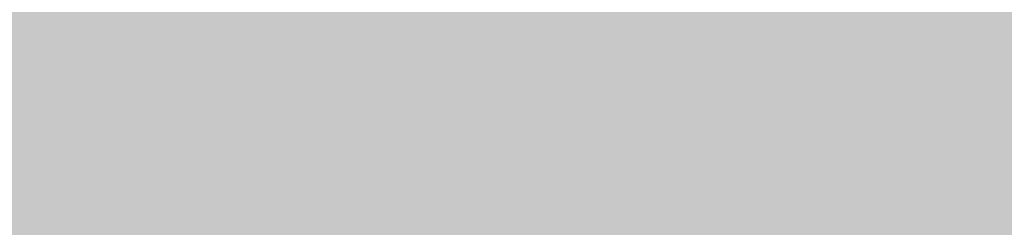
# Model space of a CAD drawing. Units: feet. Extents: x 3168 to 4724, y 827 to 1477.
# Tile 51 of 256: x 3273.0722 to 3273.13944, y 1099.00068 to 1099.01485. Entities that reach past the tile are written whole.
import ezdxf

# ---------------------------------------------------------------- set-up
doc = ezdxf.new("R2010")
doc.units = ezdxf.units.FT
doc.layers.add('A-ELEV', color=7, linetype='Continuous', lineweight=35)
doc.layers.add('A-ELEV-PATT', color=8, linetype='Continuous', lineweight=13)

msp = doc.modelspace()

# ---------------------------------------------------------------- hatches: boundary and pattern name
at = {"layer": 'A-ELEV-PATT'}
h = msp.add_hatch(color=256, dxfattribs=at)
h.dxf.hatch_style = 1
edge = h.paths.add_edge_path()
edge.add_ellipse((3552.905762, 979.220141), major_axis=(36.744924, 0), ratio=0.484848485, start_angle=0, end_angle=360)
edge = h.paths.add_edge_path()
edge.add_ellipse((3559.891637, 929.252282), major_axis=(36.744924, 0), ratio=0.484848485, start_angle=0, end_angle=360)
edge = h.paths.add_edge_path()
edge.add_line((3299.31681, 1198.606081), (3479.916714, 1198.606081))
edge.add_line((3479.916714, 1198.606081), (3479.916714, 1209.86857))
edge.add_spline(control_points=[(3479.916714, 1209.86857), (3464.301157, 1209.86857), (3448.685601, 1209.86857), (3410.949139, 1209.86857), (3388.828234, 1209.86857), (3355.646876, 1209.86857), (3344.586423, 1209.86857), (3327.995745, 1209.86857), (3322.465518, 1209.86857), (3314.170179, 1209.86857), (3311.405066, 1209.86857), (3307.257396, 1209.86857), (3305.874839, 1209.86857), (3303.801005, 1209.86857), (3303.109726, 1209.86857), (3302.072809, 1209.86857), (3301.72717, 1209.86857), (3301.208711, 1209.86857), (3301.035891, 1209.86857), (3300.776662, 1209.86857), (3300.690252, 1209.86857), (3300.560638, 1209.86857), (3300.517433, 1209.86857), (3300.452625, 1209.86857), (3300.431023, 1209.86857), (3300.398619, 1209.86857), (3300.387818, 1209.86857), (3300.366216, 1209.86857), (3300.345676, 1209.86857), (3300.345548, 1209.86857), (3300.345505, 1209.86857), (3300.343304, 1209.86857), (3300.341146, 1209.868571), (3300.337909, 1209.868571), (3300.33683, 1209.868572), (3300.333942, 1209.868573), (3300.332133, 1209.868574), (3300.325515, 1209.868577), (3300.320706, 1209.868581), (3300.310925, 1209.868592), (3300.305952, 1209.868598), (3300.290511, 1209.868623), (3300.280045, 1209.868646), (3300.232425, 1209.868777), (3300.195298, 1209.868954), (3299.951068, 1209.870608), (3299.744824, 1209.874326), (3299.436827, 1209.883257), (3299.334389, 1209.886792), (3299.181079, 1209.89292), (3299.130033, 1209.895099), (3298.652217, 1209.916801), (3298.22946, 1209.945718), (3297.601631, 1210.002367), (3297.393404, 1210.023464), (3297.082652, 1210.058309), (3296.979332, 1210.070458), (3296.292954, 1210.154861), (3295.718148, 1210.243356), (3294.868717, 1210.39885), (3294.5877, 1210.454478), (3294.169341, 1210.543349), (3294.030415, 1210.573878), (3291.707149, 1211.1012), (3289.65359, 1211.813435), (3285.776259, 1213.563988), (3283.95141, 1214.603478), (3280.512159, 1216.98008), (3278.897241, 1218.317592), (3276.379914, 1220.829489), (3275.416042, 1221.917738), (3274.039342, 1223.7077), (3273.581043, 1224.349535), (3273.143228, 1225.016316)], knot_values=[39.119033, 39.119033, 39.119033, 39.119033, 39.286353, 39.286353, 39.523379, 39.523379, 39.641892, 39.641892, 39.701148, 39.701148, 39.730777, 39.730777, 39.745591, 39.745591, 39.752998, 39.752998, 39.756701, 39.756701, 39.758553, 39.758553, 39.759479, 39.759479, 39.759942, 39.759942, 39.760173, 39.760173, 39.760289, 39.760289, 39.760405, 39.760405, 39.760463, 39.760463, 39.763389, 39.763389, 39.764851, 39.764851, 39.767304, 39.767304, 39.773825, 39.773825, 39.78057, 39.78057, 39.79477, 39.79477, 39.845194, 39.845194, 40.126715, 40.126715, 40.267476, 40.267476, 40.337856, 40.337856, 40.927023, 40.927023, 41.221606, 41.221606, 41.368898, 41.368898, 42.202622, 42.202622, 42.619485, 42.619485, 42.827916, 42.827916, 46.118323, 46.118323, 49.408731, 49.408731, 52.699139, 52.699139, 54.927489, 54.927489, 56.104228, 56.104228, 56.104228, 56.104228], weights=[1, 1, 1, 1, 1, 1, 1, 1, 1, 1, 1, 1, 1, 1, 1, 1, 1, 1, 1, 1, 1, 1, 1, 1, 1, 1, 1, 1, 1, 1, 1, 1, 1, 1, 1, 1, 1, 1, 1, 1, 1, 1, 1, 1, 1, 1, 1, 1, 1, 1, 1, 1, 1, 1, 1, 1, 1, 1, 1, 1, 1, 1, 1, 1, 1, 1, 1, 1, 1, 1, 1, 1, 1, 1], degree=3, periodic=0)
edge.add_line((3273.143228, 1225.016316), (3273.143228, 1099.016316))
edge.add_line((3273.143228, 1099.016316), (3299.31681, 1099.016316))
edge.add_line((3299.31681, 1099.016316), (3299.31681, 1198.606081))
edge = h.paths.add_edge_path()
edge.add_line((3304.758443, 1324.15806), (3479.916714, 1324.15806))
edge.add_line((3479.916714, 1324.15806), (3479.916714, 1335.714618))
edge.add_line((3479.916714, 1335.714618), (3269.161628, 1335.714618))
edge.add_spline(control_points=[(3269.161628, 1335.714618), (3264.024231, 1335.714618), (3258.364118, 1328.958189), (3259.264311, 1323.900274)], knot_values=[0, 0, 0, 0, 15.412191, 15.412191, 15.412191, 15.412191], degree=3, periodic=0)
edge.add_line((3259.264311, 1323.900274), (3265.516849, 1288.769135))
edge.add_line((3265.516849, 1288.769135), (3275.265103, 1261.545626))
edge.add_line((3275.265103, 1261.545626), (3304.758443, 1261.545626))
edge.add_line((3304.758443, 1261.545626), (3304.758443, 1324.15806))
h = msp.add_hatch(color=256, dxfattribs=at)
h.dxf.hatch_style = 1
h.paths.add_polyline_path([(3384.525247, 1099.016316), (3335.029168, 1099.016316), (3299.31681, 1099.016316), (3273.143228, 1099.016316), (3217.565364, 1099.016316), (3168.069285, 827.11626), (3335.029168, 827.11626)])

# ---------------------------------------------------------------- linework, layer by layer
at = {"layer": 'A-ELEV'}
msp.add_open_spline([(3808.5202, 1099.016316), (3808.5202, 1141.413235), (3808.5202, 1183.810154), (3808.5202, 1226.635324), (3808.5202, 1227.063576), (3808.5202, 1227.491828), (3811.491871, 1248.994673), (3814.463542, 1270.497518), (3817.46523, 1292.217564), (3817.495247, 1292.434764), (3817.525264, 1292.651964), (3817.572801, 1310.106748), (3817.620339, 1327.561532), (3817.667877, 1345.016316), (3817.667877, 1345.457962), (3817.667877, 1345.899608), (3817.667877, 1346.456047), (3817.667877, 1346.57084), (3817.667877, 1346.752887), (3817.667877, 1346.820142), (3817.667877, 1346.93487), (3817.667877, 1346.982345), (3817.667877, 1347.038587), (3817.667877, 1347.047356), (3817.667877, 1347.073661), (3817.667877, 1347.059303), (3817.667877, 1347.061545), (3817.667876, 1347.062667), (3817.667875, 1347.066031), (3817.667874, 1347.068274), (3817.66787, 1347.075001), (3817.667866, 1347.079486), (3817.667849, 1347.092937), (3817.667833, 1347.101902), (3817.667766, 1347.12879), (3817.667699, 1347.146705), (3817.667432, 1347.200421), (3817.667165, 1347.236192), (3817.6661, 1347.343385), (3817.665038, 1347.414686), (3817.660812, 1347.628095), (3817.656608, 1347.769708), (3817.63997, 1348.192487), (3817.623509, 1348.471586), (3817.559094, 1349.300067), (3817.496121, 1349.840588), (3817.255432, 1351.424156), (3817.026318, 1352.428785), (3816.306871, 1354.888914), (3815.743745, 1356.268727), (3814.463959, 1358.81921), (3813.746413, 1359.990968), (3812.195838, 1362.172343), (3811.362245, 1363.182124), (3809.588836, 1365.069009), (3808.648816, 1365.946105), (3806.654262, 1367.579616), (3805.599702, 1368.336154), (3803.352891, 1369.722327), (3802.160535, 1370.352386), (3799.600813, 1371.453586), (3798.232688, 1371.925481), (3795.280084, 1372.634624), (3793.693148, 1372.872068), (3791.869441, 1372.92648), (3791.740861, 1372.92922), (3791.353371, 1372.934101), (3791.092707, 1372.932901), (3790.304116, 1372.915068), (3789.769543, 1372.884195), (3789.20919, 1372.830236), (3789.190622, 1372.828424), (3789.134892, 1372.822912), (3789.097705, 1372.819137), (3789.048445, 1372.814008), (3789.0364, 1372.812743), (3789.000256, 1372.808918), (3788.976147, 1372.806325), (3788.949405, 1372.803404), (3788.946786, 1372.803118), (3788.942567, 1372.802655), (3788.940967, 1372.80248), (3788.938572, 1372.802217), (3788.937777, 1372.802129), (3788.935391, 1372.801867), (3788.867535, 1372.794402), (3788.756866, 1372.782228), (3788.701532, 1372.776141), (3788.53553, 1372.75788), (3788.424861, 1372.745707), (3788.092856, 1372.709185), (3787.871519, 1372.684837), (3787.207509, 1372.611793), (3786.764835, 1372.563097), (3785.436814, 1372.417009), (3784.551467, 1372.319617), (3781.895425, 1372.027442), (3780.12473, 1371.832658), (3774.812646, 1371.248307), (3771.271256, 1370.858739), (3760.647088, 1369.690037), (3753.56431, 1368.910902), (3732.315973, 1366.573498), (3718.150416, 1365.015228), (3694.006758, 1362.359326), (3684.028657, 1361.261694), (3674.050557, 1360.164062), (3664.600662, 1360.164062), (3655.150767, 1360.164062), (3626.801081, 1360.164062), (3607.901291, 1360.164062), (3551.20192, 1360.164062), (3513.40234, 1360.164062), (3467.725182, 1360.164062), (3459.847604, 1360.164062), (3436.214873, 1360.164062), (3420.459718, 1360.164062), (3373.194255, 1360.164062), (3341.683946, 1360.164062), (3302.848162, 1360.164062), (3295.522686, 1360.164062), (3286.038292, 1360.164062), (3283.879372, 1360.164062), (3277.402613, 1360.164062), (3273.084773, 1360.164062), (3267.732851, 1360.164062), (3266.698768, 1360.164062), (3263.59652, 1360.164062), (3261.528355, 1360.164062), (3259.236943, 1360.164062), (3259.013697, 1360.164062), (3258.343958, 1360.164062), (3257.897466, 1360.164062), (3257.430998, 1360.164062), (3257.411022, 1360.164062), (3257.370573, 1360.164062), (3257.37547, 1360.164062), (3257.374598, 1360.164062), (3257.373937, 1360.164062), (3257.371956, 1360.164062), (3257.370635, 1360.164061), (3257.366673, 1360.16406), (3257.364032, 1360.164059), (3257.356109, 1360.164053), (3257.350828, 1360.164047), (3257.334987, 1360.164023), (3257.32443, 1360.163998), (3257.292769, 1360.163899), (3257.271676, 1360.163799), (3257.208439, 1360.163398), (3257.166337, 1360.162995), (3257.040206, 1360.161388), (3256.956349, 1360.159783), (3256.705504, 1360.153393), (3256.53924, 1360.147036), (3256.04357, 1360.121916), (3255.717296, 1360.097102), (3254.752446, 1360.000481), (3254.127968, 1359.906513), (3252.180067, 1359.525332), (3250.941574, 1359.143991), (3248.670175, 1358.24329), (3247.635739, 1357.723834), (3245.732632, 1356.603471), (3244.863388, 1356.00206), (3243.253108, 1354.742865), (3242.511972, 1354.084731), (3240.751052, 1352.344781), (3239.800961, 1351.229574), (3238.087769, 1348.87244), (3237.324685, 1347.630355), (3235.98251, 1344.971632), (3235.402205, 1343.554907), (3234.591081, 1340.815458), (3234.310882, 1339.54355), (3233.97649, 1336.802561), (3233.922113, 1335.330877), (3234.148916, 1332.591269), (3234.349529, 1331.367201), (3234.719893, 1329.999367), (3234.752423, 1329.883362), (3234.853619, 1329.534797), (3234.925892, 1329.301685), (3235.024836, 1329.002552), (3235.046924, 1328.936928), (3235.077639, 1328.847239), (3235.085924, 1328.823198), (3235.110939, 1328.751064), (3235.127828, 1328.702962), (3235.147992, 1328.646242), (3235.151059, 1328.637632), (3235.156096, 1328.623526), (3235.158061, 1328.61803), (3235.160209, 1328.61203), (3235.165612, 1328.596943), (3235.180099, 1328.556486), (3235.190263, 1328.528101), (3235.220756, 1328.442946), (3235.241084, 1328.386176), (3235.302069, 1328.215865), (3235.342726, 1328.102325), (3235.464696, 1327.761704), (3235.54601, 1327.534623), (3235.78995, 1326.853381), (3235.952577, 1326.39922), (3236.440459, 1325.036736), (3236.765713, 1324.128414), (3237.741475, 1321.403446), (3238.391983, 1319.586801), (3240.343508, 1314.136866), (3241.644525, 1310.503576), (3245.547574, 1299.603706), (3248.149607, 1292.337126), (3255.955706, 1270.537385), (3261.159772, 1256.004225), (3267.387618, 1238.612001), (3268.411397, 1235.752937), (3269.510378, 1232.683864), (3269.585579, 1232.473854), (3269.706612, 1232.135851), (3269.752444, 1232.007857), (3269.827329, 1231.79873), (3269.856382, 1231.717595), (3269.906325, 1231.578122), (3269.927215, 1231.519782), (3269.972468, 1231.393406), (3269.996831, 1231.325368), (3270.026503, 1231.242506), (3270.031811, 1231.227681), (3270.040282, 1231.204024), (3270.039224, 1231.206979), (3270.039359, 1231.206601), (3270.039427, 1231.206412), (3270.03963, 1231.205846), (3270.039765, 1231.205468), (3270.040171, 1231.204335), (3270.040442, 1231.203579), (3270.041254, 1231.201313), (3270.041796, 1231.199802), (3270.04342, 1231.195269), (3270.044504, 1231.192248), (3270.047756, 1231.183185), (3270.049926, 1231.177145), (3270.056442, 1231.159028), (3270.060793, 1231.146957), (3270.073867, 1231.110761), (3270.082613, 1231.086656), (3270.108936, 1231.014413), (3270.1266, 1230.96635), (3270.179934, 1230.822457), (3270.215947, 1230.726923), (3270.325323, 1230.441508), (3270.400026, 1230.252811), (3270.629249, 1229.691444), (3270.788883, 1229.323501), (3271.286488, 1228.238319), (3271.6431, 1227.539755), (3272.775859, 1225.515277), (3273.614169, 1224.260502), (3275.416042, 1221.917738), (3276.379914, 1220.829489), (3278.897241, 1218.317592), (3280.512159, 1216.98008), (3283.95141, 1214.603478), (3285.776259, 1213.563988), (3289.65359, 1211.813435), (3291.707149, 1211.1012), (3294.030415, 1210.573878), (3294.169341, 1210.543349), (3294.5877, 1210.454478), (3294.868717, 1210.39885), (3295.718148, 1210.243356), (3296.292954, 1210.154861), (3296.979332, 1210.070458), (3297.082652, 1210.058309), (3297.393404, 1210.023464), (3297.601631, 1210.002367), (3298.22946, 1209.945718), (3298.652217, 1209.916801), (3299.130033, 1209.895099), (3299.181079, 1209.89292), (3299.334389, 1209.886792), (3299.436827, 1209.883257), (3299.744824, 1209.874326), (3299.951068, 1209.870608), (3300.195298, 1209.868954), (3300.232425, 1209.868777), (3300.280045, 1209.868646), (3300.290511, 1209.868623), (3300.305952, 1209.868598), (3300.310925, 1209.868592), (3300.320706, 1209.868581), (3300.325515, 1209.868577), (3300.332133, 1209.868574), (3300.333942, 1209.868573), (3300.33683, 1209.868572), (3300.337909, 1209.868571), (3300.341146, 1209.868571), (3300.343304, 1209.86857), (3300.345505, 1209.86857), (3300.345548, 1209.86857), (3300.345676, 1209.86857), (3300.366216, 1209.86857), (3300.387818, 1209.86857), (3300.398619, 1209.86857), (3300.431023, 1209.86857), (3300.452625, 1209.86857), (3300.517433, 1209.86857), (3300.560638, 1209.86857), (3300.690252, 1209.86857), (3300.776662, 1209.86857), (3301.035891, 1209.86857), (3301.208711, 1209.86857), (3301.72717, 1209.86857), (3302.072809, 1209.86857), (3303.109726, 1209.86857), (3303.801005, 1209.86857), (3305.874839, 1209.86857), (3307.257396, 1209.86857), (3311.405066, 1209.86857), (3314.170179, 1209.86857), (3322.465518, 1209.86857), (3327.995745, 1209.86857), (3344.586423, 1209.86857), (3355.646876, 1209.86857), (3388.828234, 1209.86857), (3410.949139, 1209.86857), (3477.311855, 1209.86857), (3521.553665, 1209.86857), (3566.836184, 1209.86857), (3567.876892, 1209.86857), (3570.999017, 1209.86857), (3573.080433, 1209.86857), (3575.781396, 1209.86857), (3576.400943, 1209.86857), (3577.295821, 1209.86857), (3577.571152, 1209.86857), (3578.397146, 1209.86857), (3578.947808, 1209.86857), (3579.756491, 1209.86857), (3580.014511, 1209.86857), (3580.342737, 1209.86857), (3580.326865, 1209.86857), (3580.32717, 1209.86857), (3580.327323, 1209.86857), (3580.327781, 1209.86857), (3580.328086, 1209.86857), (3580.329002, 1209.86857), (3580.329613, 1209.86857), (3580.331445, 1209.86857), (3580.332667, 1209.86857), (3580.336332, 1209.868569), (3580.338775, 1209.868567), (3580.346107, 1209.868563), (3580.350995, 1209.868558), (3580.365663, 1209.86854), (3580.375445, 1209.868522), (3580.404801, 1209.868449), (3580.424386, 1209.868376), (3580.483183, 1209.868085), (3580.522437, 1209.867793), (3580.640361, 1209.866624), (3580.719195, 1209.865454), (3580.956315, 1209.860766), (3581.115222, 1209.85607), (3581.594164, 1209.83723), (3581.916419, 1209.818331), (3582.889947, 1209.742428), (3583.547986, 1209.666169), (3585.531827, 1209.360617), (3586.867216, 1209.053886), (3589.471545, 1208.252472), (3590.740241, 1207.757852), (3591.995451, 1207.158802), (3592.057809, 1207.12874), (3592.244242, 1207.037954), (3592.367676, 1206.976632), (3592.73528, 1206.790359), (3592.976752, 1206.663101), (3593.244539, 1206.516441), (3593.274731, 1206.499825), (3593.365115, 1206.449839), (3593.425113, 1206.416333), (3593.604314, 1206.315285), (3593.722725, 1206.247211), (3593.857212, 1206.168398), (3593.874362, 1206.158319), (3593.925741, 1206.128041), (3593.959899, 1206.107798), (3594.062086, 1206.046899), (3594.129827, 1206.006074), (3594.208436, 1205.958171), (3594.219683, 1205.951304), (3594.253391, 1205.930686), (3594.275819, 1205.916917), (3594.342972, 1205.875536), (3594.387563, 1205.847853), (3594.433616, 1205.81905), (3594.435256, 1205.818024), (3594.440175, 1205.814946), (3594.443453, 1205.812894), (3594.447123, 1205.810594), (3594.447516, 1205.810348), (3594.448695, 1205.80961), (3594.449481, 1205.809117), (3594.450366, 1205.808562), (3594.450466, 1205.8085), (3594.4506, 1205.808415), (3594.467399, 1205.797887), (3594.493269, 1205.781674), (3594.506204, 1205.773568), (3594.545008, 1205.749248), (3594.570878, 1205.733035), (3594.648487, 1205.684396), (3594.700226, 1205.651969), (3594.855444, 1205.554691), (3594.958922, 1205.489839), (3595.269357, 1205.295282), (3595.476314, 1205.165577), (3596.097185, 1204.776463), (3596.511099, 1204.517054), (3597.752841, 1203.738826), (3598.580669, 1203.220007), (3601.064152, 1201.663551), (3602.719807, 1200.625914), (3607.686774, 1197.513002), (3610.998085, 1195.437727), (3620.932018, 1189.211903), (3627.55464, 1185.061354), (3647.422507, 1172.609707), (3660.667751, 1164.308608), (3700.403484, 1139.405313), (3726.893973, 1122.803116), (3757.205715, 1103.806052), (3761.02697, 1101.411184), (3764.848224, 1099.016316), (3745.328271, 1099.016316), (3725.808319, 1099.016316), (3706.288366, 1099.016316), (3706.288366, 1108.453237), (3706.288366, 1117.890158), (3706.288366, 1127.327079), (3710.750754, 1127.327079), (3715.213143, 1127.327079), (3719.675531, 1127.327079)], degree=3, knots=[0, 0, 0, 0, 0.982037, 0.982037, 0.991957, 0.991957, 0.991957, 1.966522, 1.966522, 1.976367, 1.976367, 1.976367, 2.976367, 2.976367, 2.976367, 3.00169, 3.00169, 3.008272, 3.008272, 3.012129, 3.012129, 3.014851, 3.014851, 3.015353, 3.015353, 3.016359, 3.016359, 3.017365, 3.017365, 3.019376, 3.019376, 3.023398, 3.023398, 3.031442, 3.031442, 3.047531, 3.047531, 3.079708, 3.079708, 3.144063, 3.144063, 3.272772, 3.272772, 3.53019, 3.53019, 4.045026, 4.045026, 5.074698, 5.074698, 6.700878, 6.700878, 8.327058, 8.327058, 9.953238, 9.953238, 11.579418, 11.579418, 13.205598, 13.205598, 14.831778, 14.831778, 16.457958, 16.457958, 18.084138, 18.084138, 18.206872, 18.206872, 18.45234, 18.45234, 18.943275, 18.943275, 18.960093, 18.960093, 18.993729, 18.993729, 19.00461, 19.00461, 19.026374, 19.026374, 19.028737, 19.028737, 19.03018, 19.03018, 19.030897, 19.030897, 19.032332, 19.032332, 19.033766, 19.033766, 19.036636, 19.036636, 19.042374, 19.042374, 19.053851, 19.053851, 19.076805, 19.076805, 19.122714, 19.122714, 19.21453, 19.21453, 19.398163, 19.398163, 19.765429, 19.765429, 20.024128, 20.024128, 20.024128, 20.092031, 20.092031, 20.227836, 20.227836, 20.499446, 20.499446, 20.556051, 20.556051, 20.66926, 20.66926, 20.895678, 20.895678, 20.948316, 20.948316, 20.963829, 20.963829, 20.994855, 20.994855, 21.002285, 21.002285, 21.017146, 21.017146, 21.01875, 21.01875, 21.021959, 21.021959, 21.022102, 21.022102, 21.022249, 21.022249, 21.022708, 21.022708, 21.023627, 21.023627, 21.025464, 21.025464, 21.029138, 21.029138, 21.036486, 21.036486, 21.051183, 21.051183, 21.080575, 21.080575, 21.139361, 21.139361, 21.256932, 21.256932, 21.492073, 21.492073, 21.962356, 21.962356, 23.01002, 23.01002, 24.057684, 24.057684, 25.105348, 25.105348, 26.153011, 26.153011, 27.776787, 27.776787, 29.400562, 29.400562, 31.024337, 31.024337, 32.278801, 32.278801, 33.533265, 33.533265, 34.467568, 34.467568, 34.553971, 34.553971, 34.726776, 34.726776, 34.775309, 34.775309, 34.793079, 34.793079, 34.82862, 34.82862, 34.834979, 34.834979, 34.839039, 34.839039, 34.839411, 34.839411, 34.840285, 34.840285, 34.842034, 34.842034, 34.845531, 34.845531, 34.852525, 34.852525, 34.866512, 34.866512, 34.894488, 34.894488, 34.950439, 34.950439, 35.062342, 35.062342, 35.286147, 35.286147, 35.733758, 35.733758, 35.821815, 35.821815, 35.828283, 35.828283, 35.832225, 35.832225, 35.834724, 35.834724, 35.836521, 35.836521, 35.838617, 35.838617, 35.839073, 35.839073, 35.839345, 35.839345, 35.839617, 35.839617, 35.840161, 35.840161, 35.841249, 35.841249, 35.843425, 35.843425, 35.847778, 35.847778, 35.856482, 35.856482, 35.873891, 35.873891, 35.908709, 35.908709, 35.978345, 35.978345, 36.117617, 36.117617, 36.396161, 36.396161, 36.953248, 36.953248, 38.067423, 38.067423, 40.295772, 40.295772, 42.524122, 42.524122, 45.81453, 45.81453, 49.104937, 49.104937, 52.395345, 52.395345, 52.603776, 52.603776, 53.020639, 53.020639, 53.854363, 53.854363, 54.001655, 54.001655, 54.296238, 54.296238, 54.885405, 54.885405, 54.955785, 54.955785, 55.096546, 55.096546, 55.378067, 55.378067, 55.42849, 55.42849, 55.442691, 55.442691, 55.449436, 55.449436, 55.455957, 55.455957, 55.458409, 55.458409, 55.459872, 55.459872, 55.462798, 55.462798, 55.462856, 55.462856, 55.462972, 55.462972, 55.463088, 55.463088, 55.463319, 55.463319, 55.463782, 55.463782, 55.464708, 55.464708, 55.46656, 55.46656, 55.470263, 55.470263, 55.47767, 55.47767, 55.492484, 55.492484, 55.522112, 55.522112, 55.581369, 55.581369, 55.699882, 55.699882, 55.936907, 55.936907, 56.410959, 56.410959, 56.42211, 56.42211, 56.444413, 56.444413, 56.451051, 56.451051, 56.454001, 56.454001, 56.459901, 56.459901, 56.462666, 56.462666, 56.463418, 56.463418, 56.464171, 56.464171, 56.465675, 56.465675, 56.468684, 56.468684, 56.474702, 56.474702, 56.486738, 56.486738, 56.51081, 56.51081, 56.558955, 56.558955, 56.655243, 56.655243, 56.847821, 56.847821, 57.232975, 57.232975, 58.003284, 58.003284, 59.543901, 59.543901, 62.625137, 62.625137, 68.787607, 68.787607, 74.950078, 74.950078, 75.27336, 75.27336, 75.919923, 75.919923, 77.213051, 77.213051, 77.377769, 77.377769, 77.707206, 77.707206, 78.366079, 78.366079, 78.462532, 78.462532, 78.655436, 78.655436, 79.041245, 79.041245, 79.105735, 79.105735, 79.234714, 79.234714, 79.492672, 79.492672, 79.502197, 79.502197, 79.521249, 79.521249, 79.523534, 79.523534, 79.528103, 79.528103, 79.528682, 79.528682, 79.528885, 79.528885, 79.529089, 79.529089, 79.529495, 79.529495, 79.530308, 79.530308, 79.531935, 79.531935, 79.535187, 79.535187, 79.541693, 79.541693, 79.554704, 79.554704, 79.580725, 79.580725, 79.632769, 79.632769, 79.736856, 79.736856, 79.94503, 79.94503, 80.361377, 80.361377, 80.421435, 80.421435, 80.421435, 81.421435, 81.421435, 81.421435, 82.421435, 82.421435, 82.421435, 83.421435, 83.421435, 83.421435, 83.421435], dxfattribs=at)

doc.saveas('drawing.dxf')
